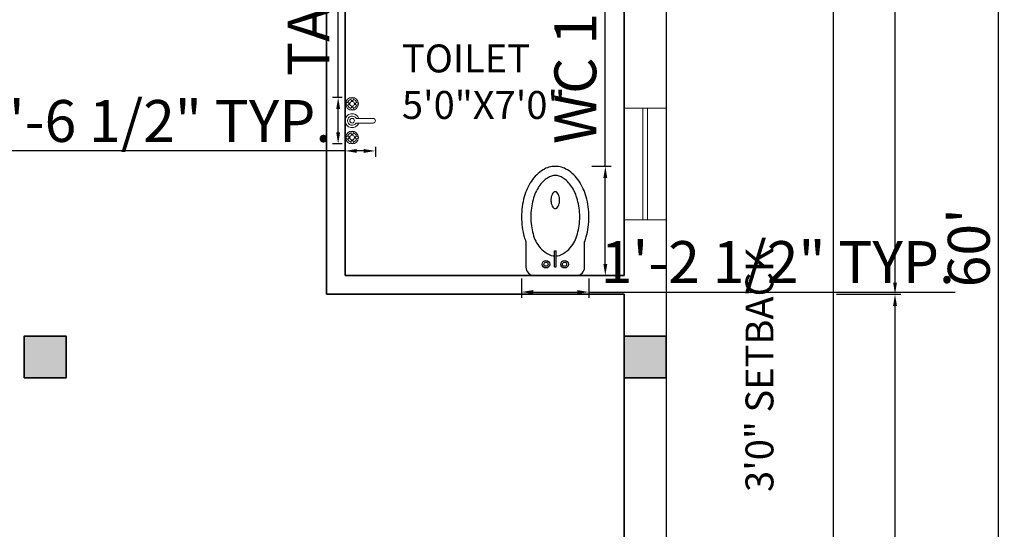
# Model space of a CAD drawing. Units: inches. Extents: x 3321 to 5237, y 11 to 1752.
# Tile 28 of 43: x 4991 to 5203, y 1287 to 1396. Entities that reach past the tile are written whole.
import ezdxf

# ---------------------------------------------------------------- set-up
doc = ezdxf.new("R2010")
doc.units = ezdxf.units.IN
for name, color, linetype, lineweight in [('A-ANNO-DIMS', 2, 'Continuous', 18), ('A-ANNO-TEXT', 7, 'Continuous', 18), ('A-AREA-IDEN', 7, 'Continuous', 18), ('A-COLS', 1, 'Continuous', 35), ('A-FLOR-EDGE', 7, 'Continuous', 25), ('A-GLAZ', 5, 'Continuous', 18), ('A-WALL', 7, 'Continuous', 35), ('C-PROP', 7, 'Continuous', 30), ('Сантехника', 7, 'Continuous', 18)]:
    doc.layers.add(name, color=color, linetype=linetype, lineweight=lineweight)
doc.layers.add('SANTEH', color=7, linetype='Continuous')
doc.styles.get("Standard").update_dxf_attribs({"font": 'arial.ttf'})
doc.dimstyles.new('ISO-25', dxfattribs={"dimtxt": 9, "dimasz": 2.5, "dimexe": 1.25, "dimexo": 0.625, "dimtad": 1, "dimdec": 1, "dimlunit": 3, "dimtxsty": 'Standard', "dimcen": 2.5, "dimclrd": 4, "dimclre": 4, "dimclrt": 256, "dimadec": 0, "dimazin": 0, "dimtfac": 1, "dimtdec": 1, "dimtmove": 0, "dimatfit": 3, "dimfxl": 1, "dimarcsym": 0})

# ---------------------------------------------------------------- blocks, each defined once
blk = doc.blocks.new('*D21')
at = {"layer": 'A-ANNO-DIMS', "color": 0, "lineweight": -2, "transparency": 16777216}
for p, q in [((5166.71, 1337.34), (5180.54, 1337.34)), ((5179.29, 1183.84), (5179.29, 1334.84)), ((5166.71, 1181.34), (5180.54, 1181.34))]:
    blk.add_line(p, q, dxfattribs=at)
at = {"layer": 'A-ANNO-DIMS', "color": 0, "transparency": 16777216}
for points in [[(5178.88, 1334.84), (5179.71, 1334.84), (5179.29, 1337.34)], [(5178.88, 1183.84), (5179.71, 1183.84), (5179.29, 1181.34)]]:
    blk.add_solid(points, dxfattribs=at)
at = {"layer": 'Defpoints', "color": 0, "transparency": 16777216}
for p in [(5166.08, 1337.34), (5179.29, 1337.34), (5166.08, 1181.34)]:
    blk.add_point(p, dxfattribs=at)
at = {"layer": 'A-ANNO-DIMS', "color": 0, "transparency": 16777216, "insert": (5174.07, 1259.34), "char_height": 9, "attachment_point": 5, "rotation": 90}
blk.add_mtext("13'", dxfattribs=at)
blk = doc.blocks.new('*D22')
at = {"layer": 'A-ANNO-DIMS', "color": 0, "lineweight": -2, "transparency": 16777216}
for p, q in [((5166.71, 1687.34), (5180.54, 1687.34)), ((5179.29, 1339.84), (5179.29, 1684.84)), ((5166.71, 1337.34), (5180.54, 1337.34))]:
    blk.add_line(p, q, dxfattribs=at)
at = {"layer": 'A-ANNO-DIMS', "color": 0, "transparency": 16777216}
for points in [[(5178.88, 1684.84), (5179.71, 1684.84), (5179.29, 1687.34)], [(5178.88, 1339.84), (5179.71, 1339.84), (5179.29, 1337.34)]]:
    blk.add_solid(points, dxfattribs=at)
at = {"layer": 'Defpoints', "color": 0, "transparency": 16777216}
for p in [(5166.08, 1687.34), (5179.29, 1687.34), (5166.08, 1337.34)]:
    blk.add_point(p, dxfattribs=at)
at = {"layer": 'A-ANNO-DIMS', "color": 0, "transparency": 16777216, "insert": (5174.07, 1512.34), "char_height": 9, "attachment_point": 5, "rotation": 90}
blk.add_mtext('29\'-2"', dxfattribs=at)
blk = doc.blocks.new('K10-45')
at = {"layer": 'SANTEH'}
for p, q in [((-18.9, 83.4), (-18.9, 177.1)), ((-18.9, 177.1), (-8.9, 177.1)), ((-8.9, 83.4), (-8.9, 177.1)), ((-18.9, 83.4), (-8.9, 83.4))]:
    blk.add_line(p, q, dxfattribs=at)
for points in [[(160.3, 230.4, 0.023928), (169.9, 259.6, 0.067459), (186.1, 379, 0.067459), (169.9, 498.4, 0.079812), (127.5, 591.1, 0.107118), (58, 658.5, 0.139889), (-13.9, 679, 0.139889), (-85.8, 658.5, 0.107118), (-155.3, 591.1, 0.079812), (-197.7, 498.4, 0.067459), (-213.9, 379, 0.067459), (-197.7, 259.6, 0.023928), (-188.1, 230.4), (-188.1, 80.2, 0.414214), (-138.1, 30.2), (110.3, 30.2, 0.414214), (160.3, 80.2)], [(-39.4, 478.5, 0.052061), (-37.3, 458.3, 0.065919), (-32, 443.1, 0.104629), (-22.6, 431.5, 0.172287), (-13.9, 428.4, 0.172287), (-5.2, 431.5, 0.104629), (4.1, 443.1, 0.065919), (9.5, 458.3, 0.052061), (11.6, 478.5, 0.052061), (9.5, 498.7, 0.065919), (4.1, 513.9, 0.104629), (-5.2, 525.5, 0.172287), (-13.9, 528.6, 0.172287), (-22.6, 525.5, 0.104629), (-32, 513.9, 0.065919), (-37.3, 498.7, 0.052061)]]:
    blk.add_lwpolyline(points, format="xyb", close=True, dxfattribs=at)
blk.add_lwpolyline([(-3.9, 147), (-1.4, 147.2), (10.9, 150.3), (23, 155.1), (34.7, 161.4), (45.9, 168.8), (56.5, 177.2), (66.3, 186.2), (75.2, 195.5), (83.2, 205), (90.3, 214.7), (96.5, 224.5), (102, 234.5), (106.9, 244.7), (111.1, 255.3), (114.8, 266.2), (118.1, 277.6), (121.1, 289.3), (123.7, 301.4), (126, 313.8), (127.9, 326.5), (129.3, 339.5), (130.4, 352.6), (131.1, 365.8), (131.3, 379), (131.1, 392.2), (130.4, 405.4), (129.3, 418.5), (127.9, 431.4), (126, 444.2), (123.7, 456.6), (121.1, 468.7), (118.1, 480.4), (114.8, 491.7), (111.2, 502.6), (107.3, 513.1), (103, 523.1), (98.4, 532.7), (93.5, 541.9), (88.3, 550.7), (82.8, 559.1), (77.1, 567.1), (71, 574.6), (64.9, 581.7), (58.5, 588.3), (52.1, 594.4), (45.7, 600), (39.3, 605), (33, 609.4), (26.9, 613.2), (20.8, 616.4), (14.9, 619), (9, 621.1), (3.2, 622.7), (-2.5, 623.8), (-8.2, 624.5), (-13.9, 624.7), (-19.6, 624.5), (-25.3, 623.8), (-31, 622.7), (-36.8, 621.1), (-42.7, 619), (-48.6, 616.4), (-54.7, 613.2), (-60.9, 609.4), (-67.2, 605), (-73.5, 600), (-80, 594.4), (-86.4, 588.3), (-92.7, 581.7), (-98.9, 574.6), (-104.9, 567.1), (-110.6, 559.1), (-116.1, 550.7), (-121.3, 541.9), (-126.2, 532.7), (-130.8, 523.1), (-135.1, 513.1), (-139, 502.6), (-142.7, 491.7), (-146, 480.4), (-148.9, 468.7), (-151.5, 456.6), (-153.8, 444.2), (-155.7, 431.4), (-157.2, 418.5), (-158.2, 405.4), (-158.9, 392.2), (-159.1, 379), (-158.9, 365.8), (-158.2, 352.6), (-157.2, 339.5), (-155.7, 326.5), (-153.8, 313.8), (-151.5, 301.4), (-148.9, 289.3), (-146, 277.6), (-142.6, 266.2), (-138.9, 255.3), (-134.7, 244.7), (-129.8, 234.5), (-124.4, 224.5), (-118.1, 214.7), (-111, 205), (-103.1, 195.5), (-94.1, 186.2), (-84.3, 177.2), (-73.7, 168.8), (-62.5, 161.4), (-50.8, 155.1), (-38.7, 150.3), (-26.4, 147.2), (-23.9, 147)], dxfattribs=at)
for centre, radius in [((-69.2, 98.1), 22.4), ((41.4, 98.1), 22.4), ((-69.2, 98.1), 12.4), ((41.4, 98.1), 12.4)]:
    blk.add_circle(centre, radius, dxfattribs=at)
blk = doc.blocks.new('Faucet - Bathroom top')
for p, q in [((-4.107, 0.125), (-4.375, 0.125)), ((-3.75, 0.4788), (-3.75, 0.75)), ((-3.5, 0.482), (-3.5, 0.75)), ((-3.1461, 0.125), (-2.875, 0.125)), ((3.143, 0.125), (2.875, 0.125)), ((3.5, 0.4788), (3.5, 0.75)), ((3.75, 0.482), (3.75, 0.75)), ((4.1039, 0.125), (4.375, 0.125)), ((-4.1039, -0.125), (-4.375, -0.125)), ((-3.75, -0.4821), (-3.75, -0.75)), ((-3.5, -0.4789), (-3.5, -0.75)), ((-3.143, -0.125), (-2.875, -0.125)), ((-0.5, -0.8639), (-0.5, -4.5)), ((0.5, -4.5), (0.5, -0.8631)), ((3.1461, -0.125), (2.875, -0.125)), ((3.5, -0.4821), (3.5, -0.75)), ((3.75, -0.4789), (3.75, -0.75)), ((4.107, -0.125), (4.375, -0.125))]:
    blk.add_line(p, q)
for centre, radius in [((-3.625, 0), 1.375), ((-4.625, 0), 0.2795), ((-3.625, 0), 0.5), ((-3.625, 1), 0.2795), ((-2.625, 0), 0.2795), ((0, 0), 0.5), ((3.625, 0), 1.375), ((2.625, 0), 0.2795), ((3.625, 0), 0.5), ((3.625, 1), 0.2795), ((4.625, 0), 0.2795), ((-3.625, -1), 0.2795), ((3.625, -1), 0.2795)]:
    blk.add_circle(centre, radius)
for centre, radius, start, end in [((-3.625, 0), 1, 105.2407, 164.2093), ((-3.625, 0), 1, 16.44125, 74.07887), ((0, 0), 1.5, 289.6514, 250.3603), ((0, 0), 1, 300.3431, 239.7554), ((3.625, 0), 1, 106.12, 164.0884), ((3.625, 0), 1, 16.23422, 73.90469), ((-3.625, 0), 1, 196.2342, 253.9047), ((-3.625, 0), 1, 286.12, 344.0884), ((3.625, 0), 1, 196.4413, 254.0789), ((3.625, 0), 1, 285.2407, 344.2093), ((0, -4.5), 0.5, 180, 0)]:
    blk.add_arc(centre, radius, start, end)
blk = doc.blocks.new('*D148')
at = {"layer": 'A-ANNO-DIMS', "color": 0, "lineweight": -2, "transparency": 16777216}
for p, q in [((5166.71, 1707.34), (5202.79, 1707.34)), ((5201.54, 989.84), (5201.54, 1704.84)), ((5166.71, 987.34), (5202.79, 987.34))]:
    blk.add_line(p, q, dxfattribs=at)
at = {"layer": 'A-ANNO-DIMS', "color": 0, "transparency": 16777216}
for points in [[(5201.12, 1704.84), (5201.96, 1704.84), (5201.54, 1707.34)], [(5201.12, 989.84), (5201.96, 989.84), (5201.54, 987.34)]]:
    blk.add_solid(points, dxfattribs=at)
at = {"layer": 'Defpoints', "color": 0, "transparency": 16777216}
for p in [(5166.08, 1707.34), (5201.54, 1707.34), (5166.08, 987.34)]:
    blk.add_point(p, dxfattribs=at)
at = {"layer": 'A-ANNO-DIMS', "color": 0, "transparency": 16777216, "insert": (5196.32, 1347.34), "char_height": 9, "attachment_point": 5, "rotation": 90}
blk.add_mtext("60'", dxfattribs=at)
blk = doc.blocks.new('COL-9X9-FURN-PLAN')
h = blk.add_hatch(color=256)
h.dxf.hatch_style = 1
h.paths.add_polyline_path([(9, 9), (0, 9), (0, 0), (9, 0)])
blk.add_lwpolyline([(0, 0), (9, 0), (9, 9), (0, 9)], close=True)
blk = doc.blocks.new('WIN-24IN-9IN-WALL')
for p, q in [((9, 24), (0, 24)), ((4, 24), (4, 0)), ((5, 24), (5, 0)), ((9, 0), (0, 0))]:
    blk.add_line(p, q)
blk = doc.blocks.new('PROPERTY-40X60FT')
blk.add_line((0, 720), (0, 0))
blk = doc.blocks.new('*D197')
at = {"layer": 'A-ANNO-DIMS', "color": 4, "lineweight": -2, "transparency": 16777216}
for p, q in [((5117.01, 1364.83), (5117.01, 1476.21)), ((5114.11, 1364.83), (5118.26, 1364.83)), ((5117.01, 1343.84), (5117.01, 1362.33)), ((5114.11, 1341.34), (5118.26, 1341.34))]:
    blk.add_line(p, q, dxfattribs=at)
at = {"layer": 'A-ANNO-DIMS', "color": 4, "transparency": 16777216}
for points in [[(5116.59, 1362.33), (5117.43, 1362.33), (5117.01, 1364.83)], [(5116.59, 1343.84), (5117.43, 1343.84), (5117.01, 1341.34)]]:
    blk.add_solid(points, dxfattribs=at)
at = {"layer": 'Defpoints', "color": 0, "transparency": 16777216}
for p in [(5113.49, 1364.83), (5117.01, 1364.83), (5113.49, 1341.34)]:
    blk.add_point(p, dxfattribs=at)
at = {"layer": 'A-ANNO-DIMS', "transparency": 16777216, "insert": (5111.73, 1421.77), "char_height": 9, "attachment_point": 5, "rotation": 90}
blk.add_mtext('WC 1\'-11 1/2" TYP.', dxfattribs=at)
blk = doc.blocks.new('*D198')
at = {"layer": 'A-ANNO-DIMS', "color": 4, "lineweight": -2, "transparency": 16777216}
for p, q in [((5099, 1340.71), (5099, 1336.56)), ((5113.49, 1340.71), (5113.49, 1336.56)), ((5101.5, 1337.81), (5110.99, 1337.81)), ((5113.49, 1337.81), (5192.22, 1337.81))]:
    blk.add_line(p, q, dxfattribs=at)
at = {"layer": 'A-ANNO-DIMS', "color": 4, "transparency": 16777216}
for points in [[(5101.5, 1338.23), (5101.5, 1337.4), (5099, 1337.81)], [(5110.99, 1338.23), (5110.99, 1337.4), (5113.49, 1337.81)]]:
    blk.add_solid(points, dxfattribs=at)
at = {"layer": 'Defpoints', "color": 0, "transparency": 16777216}
for p in [(5099, 1341.34), (5113.49, 1341.34), (5113.49, 1337.81)]:
    blk.add_point(p, dxfattribs=at)
at = {"layer": 'A-ANNO-DIMS', "transparency": 16777216, "insert": (5154.1, 1343.09), "char_height": 9, "attachment_point": 5}
blk.add_mtext('1\'-2 1/2" TYP.', dxfattribs=at)
blk = doc.blocks.new('*D199')
at = {"layer": 'A-ANNO-DIMS', "color": 4, "lineweight": -2, "transparency": 16777216}
for p, q in [((5059.57, 1379.64), (5059.57, 1473.41)), ((5060.44, 1379.64), (5058.32, 1379.64)), ((5059.57, 1372.14), (5059.57, 1377.14)), ((5060.44, 1369.64), (5058.32, 1369.64))]:
    blk.add_line(p, q, dxfattribs=at)
at = {"layer": 'A-ANNO-DIMS', "color": 4, "transparency": 16777216}
for points in [[(5059.15, 1377.14), (5059.99, 1377.14), (5059.57, 1379.64)], [(5059.15, 1372.14), (5059.99, 1372.14), (5059.57, 1369.64)]]:
    blk.add_solid(points, dxfattribs=at)
at = {"layer": 'Defpoints', "color": 0, "transparency": 16777216}
for p in [(5059.57, 1379.64), (5061.07, 1379.64), (5061.07, 1369.64)]:
    blk.add_point(p, dxfattribs=at)
at = {"layer": 'A-ANNO-DIMS', "transparency": 16777216, "insert": (5054.35, 1427.77), "char_height": 9, "attachment_point": 5, "rotation": 90}
blk.add_mtext('TAP 0\'-10" TYP.', dxfattribs=at)
blk = doc.blocks.new('*D200')
at = {"layer": 'A-ANNO-DIMS', "color": 4, "lineweight": -2, "transparency": 16777216}
for p, q in [((5061.07, 1368.14), (4981.49, 1368.14)), ((5061.07, 1369.01), (5061.07, 1366.89)), ((5065.07, 1368.14), (5063.57, 1368.14)), ((5067.57, 1369.01), (5067.57, 1366.89))]:
    blk.add_line(p, q, dxfattribs=at)
at = {"layer": 'A-ANNO-DIMS', "color": 4, "transparency": 16777216}
for points in [[(5063.57, 1368.55), (5063.57, 1367.72), (5061.07, 1368.14)], [(5065.07, 1368.55), (5065.07, 1367.72), (5067.57, 1368.14)]]:
    blk.add_solid(points, dxfattribs=at)
at = {"layer": 'Defpoints', "color": 0, "transparency": 16777216}
for p in [(5061.07, 1369.64), (5067.57, 1369.64), (5061.07, 1368.14)]:
    blk.add_point(p, dxfattribs=at)
at = {"layer": 'A-ANNO-DIMS', "transparency": 16777216, "insert": (5020.03, 1373.41), "char_height": 9, "attachment_point": 5}
blk.add_mtext('0\'-6 1/2" TYP.', dxfattribs=at)

msp = doc.modelspace()

# ---------------------------------------------------------------- linework, layer by layer
at = {"layer": 'A-FLOR-EDGE'}
msp.add_line((5130.08, 1687.34), (5130.08, 1091.34), dxfattribs=at)
at = {"layer": 'A-WALL'}
for p, q in [((5057.08, 1425.34), (5057.08, 1375.34)), ((5061.08, 1425.34), (5061.08, 1341.34)), ((5121.08, 1425.34), (5121.08, 1341.34)), ((5057.08, 1375.34), (5057.08, 1337.34)), ((5061.08, 1341.34), (5121.08, 1341.34)), ((5057.08, 1337.34), (5121.08, 1337.34)), ((5121.08, 1337.34), (5121.08, 1181.34))]:
    msp.add_line(p, q, dxfattribs=at)

# ---------------------------------------------------------------- block references
at = {"layer": 'A-COLS'}
for p in [(4992.08, 1319.34), (5121.08, 1319.34)]:
    msp.add_blockref('COL-9X9-FURN-PLAN', p, dxfattribs=at)
at = {"layer": 'A-GLAZ'}
msp.add_blockref('WIN-24IN-9IN-WALL', (5121.08, 1353.34), dxfattribs=at)
at = {"layer": 'C-PROP', "rotation": 180}
msp.add_blockref('PROPERTY-40X60FT', (5166.08, 1707.34), dxfattribs=at)
at = {"layer": 'Сантехника', "rotation": 90}
msp.add_blockref('Faucet - Bathroom top', (5062.57, 1374.64), dxfattribs=at)
at = {"layer": 'Сантехника', "xscale": 0.0362080263207385, "yscale": 0.0362080263207385, "zscale": 0.0362080263207385}
msp.add_blockref('K10-45', (5106.75, 1340.24), dxfattribs=at)

# ---------------------------------------------------------------- texts
at = {"layer": 'A-ANNO-TEXT', "insert": (5147.15, 1294.84), "char_height": 6, "attachment_point": 1, "rotation": 90}
msp.add_mtext_dynamic_manual_height_columns('3\'0" SETBACK', width=97.3114, gutter_width=25, heights=[0], dxfattribs=at)
at = {"layer": 'A-AREA-IDEN', "insert": (5073.28, 1391.02), "char_height": 6, "attachment_point": 1}
msp.add_mtext_dynamic_manual_height_columns('TOILET\\P5\'0"X7\'0"', width=97.3114, gutter_width=25, heights=[0], dxfattribs=at)

# ---------------------------------------------------------------- dimensions: what is measured, and where the dimension line sits
at = {"layer": 'A-ANNO-DIMS'}
for base, p1, p2, angle, override, picture, middle in [((5201.54, 1707.34), (5166.08, 987.34), (5166.08, 1707.34), 270, {"dimclrd": 0, "dimclre": 0, "dimclrt": 0}, '*D148', (5196.32, 1347.34)), ((5179.29, 1687.34), (5166.08, 1337.34), (5166.08, 1687.34), 90, {"dimclrd": 0, "dimclre": 0, "dimclrt": 0, "dimtmove": 1}, '*D22', (5174.07, 1512.34)), ((5179.29, 1337.34), (5166.08, 1181.34), (5166.08, 1337.34), 90, {"dimclrd": 0, "dimclre": 0, "dimclrt": 0, "dimtmove": 1}, '*D21', (5174.07, 1259.34))]:
    dim = msp.add_linear_dim(base=base, p1=p1, p2=p2, angle=angle, dimstyle='ISO-25', override=override, dxfattribs=at)
    dim.commit()
    dim.dimension.update_dxf_attribs({"geometry": picture, "text_midpoint": middle})
for base, p1, p2, angle, text, picture, middle in [((5117.01, 1364.83), (5113.49, 1341.34), (5113.49, 1364.83), 90, 'WC <> TYP.', '*D197', (5111.73, 1421.77)), ((5059.57, 1379.64), (5061.07, 1369.64), (5061.07, 1379.64), 90, 'TAP <> TYP.', '*D199', (5054.35, 1427.77)), ((5061.07, 1368.14), (5067.57, 1369.64), (5061.07, 1369.64), 180, '<> TYP.', '*D200', (5020.03, 1373.41))]:
    dim = msp.add_linear_dim(base=base, p1=p1, p2=p2, angle=angle, text=text, dimstyle='ISO-25', override={"dimdec": 1, "dimlfac": 1, "dimrnd": 0, "dimzin": 1, "dimdsep": 46, "dimlunit": 4, "dimfrac": 2}, dxfattribs=at)
    dim.commit()
    dim.dimension.update_dxf_attribs({"geometry": picture, "text_midpoint": middle})
dim = msp.add_linear_dim(base=(5113.49, 1337.81), p1=(5099, 1341.34), p2=(5113.49, 1341.34), text='<> TYP.', dimstyle='ISO-25', override={"dimdec": 1, "dimlfac": 1, "dimrnd": 0, "dimzin": 1, "dimdsep": 46, "dimlunit": 4, "dimfrac": 2}, dxfattribs=at)
dim.commit()
dim.dimension.update_dxf_attribs({"geometry": '*D198', "text_midpoint": (5154.1, 1343.09)})

doc.saveas('drawing.dxf')
